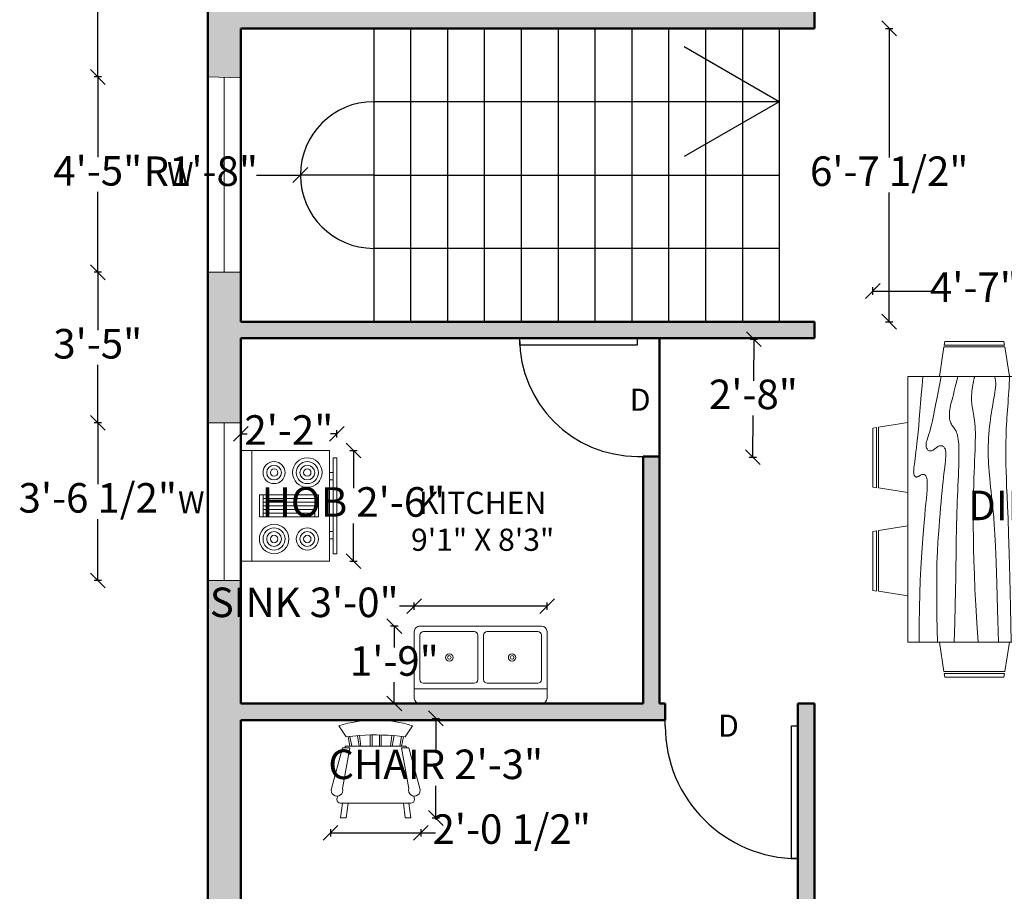
# Model space of a CAD drawing. Units: inches. Extents: x 2395 to 2921, y 528 to 1164.
# Tile 2 of 5: x 2395 to 2662, y 688 to 925. Entities that reach past the tile are written whole.
import ezdxf

# ---------------------------------------------------------------- set-up
doc = ezdxf.new("R2010")
doc.units = ezdxf.units.IN
for name, color, linetype, lineweight in [('A-ANNO-DIMS', 2, 'Continuous', 18), ('A-ANNO-TEXT', 7, 'Continuous', 18), ('A-AREA-IDEN', 7, 'Continuous', 25), ('A-DOOR', 3, 'Continuous', 25), ('A-EQPM', 9, 'Continuous', 18), ('A-FLOR-FIXT', 9, 'Continuous', 18), ('A-FLOR-STRS', 7, 'Continuous', 25), ('A-FURN', 8, 'Continuous', 18), ('A-GLAZ', 4, 'Continuous', 18), ('A-WALL', 162, 'Continuous', 50), ('A-WALL-PATT', 162, 'Continuous', 13)]:
    doc.layers.add(name, color=color, linetype=linetype, lineweight=lineweight)
doc.styles.get("Standard").update_dxf_attribs({"font": 'arial.ttf'})
doc.dimstyles.new('ISO-25', dxfattribs={"dimtxt": 8, "dimasz": 4, "dimexe": 1, "dimexo": 1, "dimtad": 0, "dimtih": 1, "dimtoh": 1, "dimlunit": 3, "dimtxsty": 'Standard', "dimblk": 'OBLIQUE', "dimcen": 2.5, "dimadec": 0, "dimazin": 0, "dimtfac": 1, "dimtmove": 0, "dimatfit": 3, "dimfxl": 1, "dimfxlon": 1, "dimarcsym": 0})

# ---------------------------------------------------------------- blocks, each defined once
blk = doc.blocks.new('*U9')
for p, q in [((0, 0), (0, -6)), ((-32, 0), (-32, -6))]:
    blk.add_line(p, q)
blk.add_lwpolyline([(0, 0), (0, 32), (-1.75, 32), (-1.75, 0)], close=True)
blk.add_arc((0, 0), 32, 90, 180)
blk = doc.blocks.new('*U5')
for p, q in [((-36, 0), (-36, 6)), ((0, 0), (0, 6))]:
    blk.add_line(p, q)
blk.add_lwpolyline([(0, 0), (0, -36), (-1.75, -36), (-1.75, 0)], close=True)
blk.add_arc((0, 0), 36, 180, 270)
blk = doc.blocks.new('Chair - Rocking')
for p, q in [((-8, -4.5), (-10, -1.5)), ((8, -4.5), (10, -1.5)), ((-7.5, -4.5), (-7, -7)), ((-6.5, -7), (-7.02225, -4.43)), ((-4.5, -7), (-4.96674, -4.19951)), ((-4, -7), (-4.40532, -4.16272)), ((-1.5, -4.05012), (-1.5, -7)), ((-1, -7), (-1, -4.05012)), ((1, -7), (1, -4.04655)), ((1.5, -4.05012), (1.5, -7)), ((4, -7), (4.40187, -4.18694)), ((4.5, -7), (4.96761, -4.19437)), ((6.5, -7), (7, -4.4057)), ((7.5, -4.5), (7, -7)), ((-9, -7.5), (-12, -18.49999)), ((-7, -7.5), (-9, -7.5)), ((-9, -18.49999), (-7, -7.5)), ((-8.23428, -6.99939), (-8.3093, -7.47958)), ((-8.23041, -7), (8.23915, -7)), ((7, -7.5), (9, -7.5)), ((9, -18.49999), (7, -7.5)), ((8.31071, -7.48854), (8.23449, -7.00073)), ((9, -7.5), (12, -18.49999)), ((-10.36644, -20.64523), (-10.5, -21.49999)), ((10.5, -21.49999), (10.3575, -20.58798)), ((-9, -22.49999), (-9.5, -26.49999)), ((0, -22.49999), (-9.5, -22.49999)), ((-8, -26.49999), (-7.5, -22.49999)), ((0, -22.49999), (9.5, -22.49999)), ((8, -26.49999), (7.5, -22.49999)), ((9, -22.49999), (9.5, -26.49999)), ((-9.5, -26.49999), (-8, -26.49999)), ((9.5, -26.49999), (8, -26.49999))]:
    blk.add_line(p, q)
for centre, radius, start, end in [((0, -34.08333), 34.08333, 72.93847, 107.0615), ((0, -68.25004), 64.25, 93.92211, 97.15267), ((0, -68.25004), 64.25, 82.84733, 93.92211), ((-10.5, -18.99999), 1.58114, 161.5651, 18.43495), ((10.5, -18.99999), 1.58114, 161.5651, 18.43495), ((-9.5, -21.49999), 1, 180, 270), ((9.5, -21.49999), 1, 270, 0)]:
    blk.add_arc(centre, radius, start, end)
blk = doc.blocks.new('Dining Set - 36 x 72 in.')
for p, q in [((-22, 27.5), (-22.1562, 26.50042)), ((-22, 27.5), (-6, 27.5)), ((-5.8437, 26.49966), (-6, 27.5)), ((6, 27.5), (5.8438, 26.50042)), ((6, 27.5), (22, 27.5)), ((22.1563, 26.49966), (22, 27.5)), ((-22.2343, 26.00059), (-23.4847, 17.99762)), ((-22.2304, 26), (-5.7608, 26)), ((-5.8416, 26.5), (-22.1534, 26.5)), ((-4.5152, 17.99762), (-5.7655, 25.99926)), ((5.7657, 26.00059), (4.5153, 17.99762)), ((5.7696, 26), (22.2392, 26)), ((22.1584, 26.5), (5.8466, 26.5)), ((23.4848, 17.99762), (22.2345, 25.99926)), ((36, 18), (-36, 18)), ((-36, 18), (-36, -18)), ((36, -18), (36, 18)), ((-45.5, 8), (-44.5004, 8.15617)), ((-44.5, -8.15843), (-44.5, 8.15338)), ((-44.0006, 8.23428), (-35.9976, 9.48474)), ((-44, 8.23041), (-44, -8.23915)), ((44.0006, 8.23428), (35.9976, 9.48474)), ((44, 8.23041), (44, -8.23915)), ((44.5, -8.15843), (44.5, 8.15338)), ((45.5, 8), (44.5005, 8.15617)), ((-45.5, 8), (-45.5, -8)), ((45.5, 8), (45.5, -8)), ((-44.4997, -8.15631), (-45.5, -8)), ((44.4997, -8.15631), (45.5, -8)), ((-35.9976, -9.48476), (-43.9993, -8.2345)), ((35.9976, -9.48476), (43.9993, -8.2345)), ((-36, -18), (36, -18)), ((-22.2343, -26.0006), (-23.4847, -17.99762)), ((-4.5152, -17.99762), (-5.7655, -25.99928)), ((5.7657, -26.0006), (4.5153, -17.99762)), ((23.4848, -17.99762), (22.2345, -25.99928)), ((-22.2304, -26), (-5.7608, -26)), ((-22, -27.5), (-22.1562, -26.50044)), ((-5.8416, -26.5), (-22.1534, -26.5)), ((-5.8437, -26.49967), (-6, -27.5)), ((5.7696, -26), (22.2392, -26)), ((6, -27.5), (5.8438, -26.50044)), ((22.1584, -26.5), (5.8466, -26.5)), ((22.1563, -26.49967), (22, -27.5)), ((-22, -27.5), (-6, -27.5)), ((6, -27.5), (22, -27.5))]:
    blk.add_line(p, q)
for points in [[(-36, 15), (-31.1772, 14.97754), (-26.8079, 14.91406), (-22.8538, 14.81543), (-19.276, 14.6875), (-16.0362, 14.53613), (-13.0957, 14.36718), (-10.4159, 14.18652), (-7.9583, 14), (-5.6904, 13.81315), (-3.6035, 13.63021), (-1.6954, 13.45508), (0.0365, 13.29166), (1.5945, 13.14388), (2.9811, 13.01562), (4.1988, 12.9108), (5.25, 12.83333), (6.1393, 12.78613), (6.8802, 12.76823), (7.4883, 12.77767), (7.9792, 12.8125), (8.3685, 12.87077), (8.6719, 12.95052), (8.9049, 13.0498), (9.0833, 13.16666), (9.2205, 13.29899), (9.3216, 13.44401), (9.3895, 13.59879), (9.4271, 13.76041), (9.4373, 13.92594), (9.4232, 14.09245), (9.3875, 14.257), (9.3333, 14.41666), (9.2638, 14.56917), (9.1836, 14.71484), (9.0975, 14.85465), (9.0104, 14.98958), (8.9272, 15.1206), (8.8529, 15.2487), (8.7922, 15.37483), (8.75, 15.5), (8.7305, 15.62467), (8.7344, 15.74739), (8.7617, 15.86621), (8.8125, 15.97916), (8.8867, 16.08431), (8.9844, 16.17968), (9.1055, 16.26334), (9.25, 16.33333), (9.4189, 16.38802), (9.6172, 16.42708), (9.8506, 16.45052), (10.125, 16.45833), (10.4463, 16.45052), (10.8203, 16.42708), (11.2529, 16.38802), (11.75, 16.33333), (12.3184, 16.26318), (12.9694, 16.17838), (13.7151, 16.07991), (14.5677, 15.96875), (15.5395, 15.84586), (16.6426, 15.71224), (17.8893, 15.56884), (19.2917, 15.41666), (20.859, 15.25667), (22.5879, 15.08984), (24.4721, 14.91715), (26.5052, 14.73958), (28.6809, 14.5581), (30.9929, 14.3737), (33.4347, 14.18733), (36, 14)], [(-36, 10), (-28.9766, 10.14274), (-23.1725, 10.20442), (-18.4241, 10.19775), (-14.5677, 10.13541), (-11.4399, 10.03011), (-8.877, 9.89453), (-6.7154, 9.74137), (-4.7917, 9.58333), (-2.9698, 9.43082), (-1.2246, 9.28515), (0.4415, 9.14534), (2.026, 9.01041), (3.5266, 8.87939), (4.9408, 8.7513), (6.266, 8.62516), (7.5, 8.5), (8.6411, 8.37549), (9.6914, 8.2539), (10.6538, 8.13818), (11.5312, 8.03125), (12.3267, 7.93603), (13.043, 7.85547), (13.6831, 7.79248), (14.25, 7.75), (14.7471, 7.7303), (15.1797, 7.73307), (15.5537, 7.75732), (15.875, 7.80208), (16.1494, 7.86637), (16.3828, 7.94922), (16.5811, 8.04964), (16.75, 8.16666), (16.8944, 8.29915), (17.0143, 8.44531), (17.1089, 8.60319), (17.1771, 8.77083), (17.218, 8.94629), (17.2305, 9.1276), (17.2137, 9.31282), (17.1667, 9.5), (17.0895, 9.6875), (16.987, 9.875), (16.8649, 10.0625), (16.7292, 10.25), (16.5856, 10.4375), (16.4401, 10.625), (16.2985, 10.8125), (16.1667, 11), (16.05, 11.18733), (15.9518, 11.3737), (15.8752, 11.5581), (15.8229, 11.73958), (15.798, 11.91715), (15.8034, 12.08984), (15.842, 12.25667), (15.9167, 12.41666), (16.0295, 12.56836), (16.1784, 12.70833), (16.3605, 12.83268), (16.5729, 12.9375), (16.8127, 13.01888), (17.0768, 13.07291), (17.3625, 13.0957), (17.6667, 13.08333), (17.9894, 13.03312), (18.3418, 12.94726), (18.7382, 12.82918), (19.1927, 12.68229), (19.7195, 12.51001), (20.3327, 12.31575), (21.0465, 12.10294), (21.875, 11.875), (22.8357, 11.63354), (23.959, 11.37304), (25.2786, 11.08618), (26.8282, 10.76562), (28.6414, 10.40405), (30.752, 9.99414), (33.1936, 9.52856), (36, 9)], [(-36, 5.5), (-30.7157, 5.3348), (-26.069, 5.20963), (-21.9946, 5.11767), (-18.4271, 5.05208), (-15.3009, 5.00602), (-12.5508, 4.97265), (-10.1112, 4.94515), (-7.9167, 4.91666), (-5.909, 4.88167), (-4.0586, 4.83984), (-2.3429, 4.79215), (-0.7396, 4.73958), (0.7739, 4.6831), (2.22, 4.6237), (3.6213, 4.56233), (5, 4.5), (6.373, 4.43782), (7.7344, 4.3776), (9.0723, 4.32129), (10.375, 4.27083), (11.6309, 4.22819), (12.8281, 4.19531), (13.9551, 4.17415), (15, 4.16666), (15.954, 4.17448), (16.819, 4.19791), (17.6001, 4.23698), (18.3021, 4.29166), (18.9299, 4.36198), (19.4883, 4.44791), (19.9823, 4.54948), (20.4167, 4.66666), (20.7969, 4.79899), (21.1302, 4.94401), (21.4245, 5.09879), (21.6875, 5.26041), (21.9271, 5.42594), (22.1511, 5.59245), (22.3672, 5.757), (22.5834, 5.91666), (22.8065, 6.06868), (23.0404, 6.21093), (23.2879, 6.34147), (23.5521, 6.45833), (23.8358, 6.55957), (24.142, 6.64323), (24.4735, 6.70735), (24.8334, 6.75), (25.2235, 6.76969), (25.642, 6.76692), (26.0858, 6.74267), (26.5521, 6.69791), (27.0379, 6.63362), (27.5404, 6.55078), (28.0565, 6.45036), (28.5834, 6.33333), (29.1242, 6.19987), (29.7071, 6.04687), (30.3661, 5.87044), (31.1354, 5.66666), (32.0493, 5.43164), (33.142, 5.16146), (34.4475, 4.85221), (36, 4.5)], [(-36, -1), (-30.7915, -0.6591), (-26.0195, -0.38216), (-21.6519, -0.16284), (-17.6563, 0.00521), (-14.0005, 0.12833), (-10.6523, 0.21289), (-7.5796, 0.26522), (-4.75, 0.29166), (-2.134, 0.29793), (0.2878, 0.28711), (2.5317, 0.26163), (4.6146, 0.22396), (6.5529, 0.17651), (8.3633, 0.12174), (10.0623, 0.06209), (11.6667, 0), (13.1899, -0.06201), (14.6341, -0.1211), (15.9982, -0.17432), (17.2813, -0.21875), (18.4823, -0.25147), (19.6003, -0.26953), (20.6343, -0.27002), (21.5834, -0.25), (22.4481, -0.20768), (23.2357, -0.14584), (23.9549, -0.06836), (24.6146, 0.02083), (25.2235, 0.11784), (25.7904, 0.21875), (26.3241, 0.31966), (26.8334, 0.41666), (27.3265, 0.50618), (27.8099, 0.58593), (28.2894, 0.65397), (28.7709, 0.70833), (29.2601, 0.74707), (29.763, 0.76823), (30.2855, 0.76985), (30.8334, 0.75), (31.4088, 0.70784), (31.9994, 0.64713), (32.589, 0.57275), (33.1615, 0.48958), (33.7008, 0.4025), (34.1908, 0.3164), (34.6153, 0.23616), (34.9584, 0.16666), (35.2099, 0.11165), (35.3848, 0.07031), (35.504, 0.04069), (35.5886, 0.02083), (35.6594, 0.00879), (35.7377, 0.0026), (35.8442, 0.00032), (36, 0)], [(-36, -6.5), (-27.1843, -6.31267), (-20.084, -6.1263), (-14.469, -5.9419), (-10.1094, -5.76042), (-6.7752, -5.58285), (-4.2363, -5.41016), (-2.2629, -5.24333), (-0.625, -5.08334), (0.8708, -4.93099), (2.2715, -4.78646), (3.5872, -4.64974), (4.8281, -4.52084), (6.0046, -4.39974), (7.127, -4.28646), (8.2053, -4.18099), (9.25, -4.08334), (10.2705, -3.99382), (11.2734, -3.91407), (12.2647, -3.84603), (13.25, -3.79167), (14.2354, -3.75293), (15.2266, -3.73177), (16.2295, -3.73015), (17.25, -3.75), (18.2912, -3.79248), (19.3451, -3.85547), (20.4009, -3.93604), (21.4479, -4.03125), (22.4754, -4.13819), (23.4727, -4.25391), (24.4289, -4.37549), (25.3334, -4.5), (26.1785, -4.62492), (26.9694, -4.74935), (27.7145, -4.87281), (28.4219, -4.99479), (29.1, -5.11483), (29.7572, -5.23242), (30.4016, -5.34709), (31.0417, -5.45834), (31.6837, -5.56437), (32.3262, -5.65821), (32.9658, -5.73153), (33.599, -5.77604), (34.2224, -5.78345), (34.8327, -5.74545), (35.4264, -5.65373), (36, -5.5)], [(-36, -10), (-26.4022, -9.81299), (-18.4675, -9.62891), (-11.9839, -9.45069), (-6.7396, -9.28125), (-2.5226, -9.12354), (0.8789, -8.98047), (3.6769, -8.85498), (6.0833, -8.75), (8.2767, -8.66765), (10.3021, -8.60677), (12.1712, -8.56543), (13.8958, -8.54167), (15.4876, -8.53353), (16.9583, -8.53907), (18.3197, -8.55632), (19.5834, -8.58334), (20.7616, -8.61841), (21.8685, -8.66081), (22.9188, -8.71004), (23.9271, -8.76563), (24.9081, -8.82707), (25.8763, -8.89388), (26.8465, -8.96558), (27.8334, -9.04167), (28.8474, -9.12118), (29.8828, -9.20117), (30.93, -9.27824), (31.9792, -9.34896), (33.0205, -9.40991), (34.0443, -9.45768), (35.0407, -9.48885), (36, -9.5)], [(-36, -14.5), (-30.0881, -14.33513), (-25.0332, -14.21224), (-20.7312, -14.12647), (-17.0781, -14.07292), (-13.97, -14.04671), (-11.3027, -14.04297), (-8.9724, -14.05681), (-6.875, -14.08334), (-4.9224, -14.11833), (-3.0905, -14.16016), (-1.3709, -14.20785), (0.2448, -14.26042), (1.7647, -14.3169), (3.1973, -14.3763), (4.5507, -14.43767), (5.8333, -14.5), (7.0554, -14.5621), (8.235, -14.62175), (9.3922, -14.67652), (10.5469, -14.72396), (11.7192, -14.76164), (12.929, -14.78711), (14.1965, -14.79794), (15.5417, -14.79167), (16.9933, -14.76424), (18.6152, -14.70508), (20.4804, -14.60197), (22.6615, -14.44271), (25.2312, -14.21509), (28.2624, -13.9069), (31.8277, -13.50594), (36, -13)]]:
    blk.add_lwpolyline(points)
blk = doc.blocks.new('Sink-double - 36 in top')
for p, q in [((-18, -4), (18, -4)), ((-0.75, -18.5), (-0.75, -6.5)), ((0.75, -6.5), (0.75, -18.5))]:
    blk.add_line(p, q)
for points in [[(-16.5, 0), (16.5, 0)], [(-18, -19.5), (-18, -1.5)], [(18, -1.5), (18, -19.5)], [(-16.5, -18.5), (-16.5, -6.5)], [(-15.5, -5.5), (-1.75, -5.5)], [(1.75, -5.5), (15.5, -5.5)], [(16.5, -6.5), (16.5, -18.5)], [(16.5, -21), (-16.5, -21)], [(-1.75, -19.5), (-15.5, -19.5)], [(15.5, -19.5), (1.75, -19.5)]]:
    blk.add_lwpolyline(points)
for centre, radius in [((-8.5, -12.5), 1), ((-8.5, -12.5), 0.5), ((8.5, -12.5), 1), ((8.5, -12.5), 0.5)]:
    blk.add_circle(centre, radius)
for centre, radius, start, end in [((-16.5, -1.5), 1.5, 90, 180), ((16.5, -1.5), 1.5, 0, 90), ((-15.5, -6.5), 1, 90, 180), ((-1.75, -6.5), 1, 0, 90), ((1.75, -6.5), 1, 90, 180), ((15.5, -6.5), 1, 0, 90), ((-15.5, -18.5), 1, 180, 270), ((-1.75, -18.5), 1, 270, 0), ((1.75, -18.5), 1, 180, 270), ((15.5, -18.5), 1, 270, 0), ((-16.5, -19.5), 1.5, 180, 270), ((16.5, -19.5), 1.5, 270, 0)]:
    blk.add_arc(centre, radius, start, end)
blk = doc.blocks.new('Range-Oven - 30 in top')
for p, q in [((0, -3), (30, -3)), ((12, -6), (18, -6)), ((13, -20), (13, -6)), ((14, -6), (14, -20)), ((15, -20), (15, -6)), ((16, -6), (16, -20)), ((17, -20), (17, -6)), ((18, -20), (12, -20)), ((6, -24), (6, -25)), ((8, -25), (8, -24)), ((22, -25), (22, -24)), ((24, -24), (24, -25))]:
    blk.add_line(p, q)
for points in [[(0, -24), (0, 0), (30, 0), (30, -24)], [(12, -21), (12, -5), (18, -5), (18, -21)], [(2, -26), (2, -25), (28, -25), (28, -26)]]:
    blk.add_lwpolyline(points, close=True)
for centre, radius in [((6, -9), 4), ((6, -9), 3), ((6, -9), 2), ((6, -9), 1), ((24, -9), 3), ((24, -9), 2), ((24, -9), 1), ((6, -18), 3), ((6, -18), 2), ((24, -18), 4), ((24, -18), 3), ((24, -18), 2), ((6, -18), 1), ((24, -18), 1)]:
    blk.add_circle(centre, radius)
blk = doc.blocks.new('_Oblique')
at = {"color": 0, "linetype": 'ByBlock', "lineweight": -2}
blk.add_line((-0.5, -0.5), (0.5, 0.5), dxfattribs=at)
blk = doc.blocks.new('*D30')
at = {"layer": 'A-ANNO-DIMS', "color": 0, "lineweight": -2, "transparency": 16777216}
for p, q in [((2507.01, 735.35), (2509.01, 735.35)), ((2508.01, 735.35), (2508.01, 726.62)), ((2508.01, 708.35), (2508.01, 717.09)), ((2507.01, 708.35), (2509.01, 708.35))]:
    blk.add_line(p, q, dxfattribs=at)
at = {"layer": 'Defpoints', "color": 0, "transparency": 16777216}
for p in [(2503.96, 735.35), (2508.01, 735.35), (2503.96, 708.35)]:
    blk.add_point(p, dxfattribs=at)
at = {"layer": 'A-ANNO-DIMS', "color": 0, "lineweight": -2, "transparency": 16777216, "xscale": 4, "yscale": 4, "zscale": 4}
for p, rotation in [((2508.01, 735.35), 90), ((2508.01, 708.35), 270)]:
    blk.add_blockref('_Oblique', p, dxfattribs=dict(at, rotation=rotation))
at = {"layer": 'A-ANNO-DIMS', "color": 0, "transparency": 16777216, "insert": (2508.01, 721.85), "char_height": 8, "attachment_point": 5}
blk.add_mtext('CHAIR 2\'-3"', dxfattribs=at)
blk = doc.blocks.new('*D31')
at = {"layer": 'A-ANNO-DIMS', "color": 0, "lineweight": -2, "transparency": 16777216}
for p, q in [((2479.52, 705.3), (2479.52, 703.3)), ((2503.96, 705.3), (2503.96, 703.3)), ((2479.52, 704.3), (2503.96, 704.3)), ((2503.96, 704.3), (2507.96, 704.3))]:
    blk.add_line(p, q, dxfattribs=at)
at = {"layer": 'Defpoints', "color": 0, "transparency": 16777216}
for p in [(2479.52, 708.35), (2503.96, 708.35), (2503.96, 704.3)]:
    blk.add_point(p, dxfattribs=at)
at = {"layer": 'A-ANNO-DIMS', "color": 0, "lineweight": -2, "transparency": 16777216, "xscale": 4, "yscale": 4, "zscale": 4, "rotation": 180}
blk.add_blockref('_Oblique', (2479.52, 704.3), dxfattribs=at)
at = {"layer": 'A-ANNO-DIMS', "color": 0, "lineweight": -2, "transparency": 16777216, "xscale": 4, "yscale": 4, "zscale": 4}
blk.add_blockref('_Oblique', (2503.96, 704.3), dxfattribs=at)
at = {"layer": 'A-ANNO-DIMS', "color": 0, "transparency": 16777216, "insert": (2528.6, 704.3), "char_height": 8, "attachment_point": 5}
blk.add_mtext('2\'-0 1/2"', dxfattribs=at)
blk = doc.blocks.new('*D36')
at = {"layer": 'A-ANNO-DIMS', "color": 0, "lineweight": -2, "transparency": 16777216}
for p, q in [((2694.16, 837.52), (2696.16, 837.52)), ((2695.16, 837.52), (2695.16, 796.78)), ((2695.16, 746.52), (2695.16, 787.26)), ((2694.16, 746.52), (2696.16, 746.52))]:
    blk.add_line(p, q, dxfattribs=at)
at = {"layer": 'Defpoints', "color": 0, "transparency": 16777216}
for p in [(2681.51, 837.52), (2695.16, 837.52), (2681.51, 746.52)]:
    blk.add_point(p, dxfattribs=at)
at = {"layer": 'A-ANNO-DIMS', "color": 0, "lineweight": -2, "transparency": 16777216, "xscale": 4, "yscale": 4, "zscale": 4}
for p, rotation in [((2695.16, 837.52), 90), ((2695.16, 746.52), 270)]:
    blk.add_blockref('_Oblique', p, dxfattribs=dict(at, rotation=rotation))
at = {"layer": 'A-ANNO-DIMS', "color": 0, "transparency": 16777216, "insert": (2695.16, 792.02), "char_height": 8, "attachment_point": 5}
blk.add_mtext('DINING SET 7\'-7"', dxfattribs=at)
blk = doc.blocks.new('*D37')
at = {"layer": 'A-ANNO-DIMS', "color": 0, "lineweight": -2, "transparency": 16777216}
for p, q in [((2626.51, 850.17), (2626.51, 852.17)), ((2681.51, 850.17), (2681.51, 852.17)), ((2626.51, 851.17), (2642.59, 851.17)), ((2681.51, 851.17), (2665.43, 851.17))]:
    blk.add_line(p, q, dxfattribs=at)
at = {"layer": 'Defpoints', "color": 0, "transparency": 16777216}
for p in [(2626.51, 851.17), (2626.51, 837.52), (2681.51, 837.52)]:
    blk.add_point(p, dxfattribs=at)
at = {"layer": 'A-ANNO-DIMS', "color": 0, "lineweight": -2, "transparency": 16777216, "xscale": 4, "yscale": 4, "zscale": 4, "rotation": 180}
blk.add_blockref('_Oblique', (2626.51, 851.17), dxfattribs=at)
at = {"layer": 'A-ANNO-DIMS', "color": 0, "lineweight": -2, "transparency": 16777216, "xscale": 4, "yscale": 4, "zscale": 4}
blk.add_blockref('_Oblique', (2681.51, 851.17), dxfattribs=at)
at = {"layer": 'A-ANNO-DIMS', "color": 0, "transparency": 16777216, "insert": (2654.01, 851.17), "char_height": 8, "attachment_point": 5}
blk.add_mtext('4\'-7"', dxfattribs=at)
blk = doc.blocks.new('*D38')
at = {"layer": 'A-ANNO-DIMS', "color": 0, "lineweight": -2, "transparency": 16777216}
for p, q in [((2502.19, 764.75), (2502.19, 766.75)), ((2538.19, 764.75), (2538.19, 766.75)), ((2502.19, 765.75), (2498.19, 765.75)), ((2538.19, 765.75), (2502.19, 765.75))]:
    blk.add_line(p, q, dxfattribs=at)
at = {"layer": 'Defpoints', "color": 0, "transparency": 16777216}
for p in [(2502.19, 765.75), (2502.19, 760.35), (2538.19, 760.35)]:
    blk.add_point(p, dxfattribs=at)
at = {"layer": 'A-ANNO-DIMS', "color": 0, "lineweight": -2, "transparency": 16777216, "xscale": 4, "yscale": 4, "zscale": 4, "rotation": 180}
blk.add_blockref('_Oblique', (2502.19, 765.75), dxfattribs=at)
at = {"layer": 'A-ANNO-DIMS', "color": 0, "lineweight": -2, "transparency": 16777216, "xscale": 4, "yscale": 4, "zscale": 4}
blk.add_blockref('_Oblique', (2538.19, 765.75), dxfattribs=at)
at = {"layer": 'A-ANNO-DIMS', "color": 0, "transparency": 16777216, "insert": (2472.36, 765.75), "char_height": 8, "attachment_point": 5}
blk.add_mtext('SINK 3\'-0"', dxfattribs=at)
blk = doc.blocks.new('*D39')
at = {"layer": 'A-ANNO-DIMS', "color": 0, "lineweight": -2, "transparency": 16777216}
for p, q in [((2497.79, 760.35), (2495.79, 760.35)), ((2496.79, 760.35), (2496.79, 754.56)), ((2496.79, 739.35), (2496.79, 745.14)), ((2497.79, 739.35), (2495.79, 739.35))]:
    blk.add_line(p, q, dxfattribs=at)
at = {"layer": 'Defpoints', "color": 0, "transparency": 16777216}
for p in [(2502.19, 760.35), (2496.79, 739.35), (2502.19, 739.35)]:
    blk.add_point(p, dxfattribs=at)
at = {"layer": 'A-ANNO-DIMS', "color": 0, "lineweight": -2, "transparency": 16777216, "xscale": 4, "yscale": 4, "zscale": 4}
for p, rotation in [((2496.79, 760.35), 90), ((2496.79, 739.35), 270)]:
    blk.add_blockref('_Oblique', p, dxfattribs=dict(at, rotation=rotation))
at = {"layer": 'A-ANNO-DIMS', "color": 0, "transparency": 16777216, "insert": (2496.79, 749.85), "char_height": 8, "attachment_point": 5}
blk.add_mtext('1\'-9"', dxfattribs=at)
blk = doc.blocks.new('*D40')
at = {"layer": 'A-ANNO-DIMS', "color": 0, "lineweight": -2, "transparency": 16777216}
for p, q in [((2484.7, 807.96), (2486.7, 807.96)), ((2485.7, 807.96), (2485.7, 797.73)), ((2485.7, 777.96), (2485.7, 788.2)), ((2484.7, 777.96), (2486.7, 777.96))]:
    blk.add_line(p, q, dxfattribs=at)
at = {"layer": 'Defpoints', "color": 0, "transparency": 16777216}
for p in [(2481.2, 807.96), (2485.7, 807.96), (2481.2, 777.96)]:
    blk.add_point(p, dxfattribs=at)
at = {"layer": 'A-ANNO-DIMS', "color": 0, "lineweight": -2, "transparency": 16777216, "xscale": 4, "yscale": 4, "zscale": 4}
for p, rotation in [((2485.7, 807.96), 90), ((2485.7, 777.96), 270)]:
    blk.add_blockref('_Oblique', p, dxfattribs=dict(at, rotation=rotation))
at = {"layer": 'A-ANNO-DIMS', "color": 0, "transparency": 16777216, "insert": (2485.7, 792.96), "char_height": 8, "attachment_point": 5}
blk.add_mtext('HOB 2\'-6"', dxfattribs=at)
blk = doc.blocks.new('*D41')
at = {"layer": 'A-ANNO-DIMS', "color": 0, "lineweight": -2, "transparency": 16777216}
for p, q in [((2455.2, 811.46), (2455.2, 813.46)), ((2455.2, 812.46), (2456.87, 812.46)), ((2481.2, 812.46), (2479.53, 812.46)), ((2481.2, 811.46), (2481.2, 813.46))]:
    blk.add_line(p, q, dxfattribs=at)
at = {"layer": 'Defpoints', "color": 0, "transparency": 16777216}
for p in [(2455.2, 812.46), (2455.2, 807.96), (2481.2, 807.96)]:
    blk.add_point(p, dxfattribs=at)
at = {"layer": 'A-ANNO-DIMS', "color": 0, "lineweight": -2, "transparency": 16777216, "xscale": 4, "yscale": 4, "zscale": 4, "rotation": 180}
blk.add_blockref('_Oblique', (2455.2, 812.46), dxfattribs=at)
at = {"layer": 'A-ANNO-DIMS', "color": 0, "lineweight": -2, "transparency": 16777216, "xscale": 4, "yscale": 4, "zscale": 4}
blk.add_blockref('_Oblique', (2481.2, 812.46), dxfattribs=at)
at = {"layer": 'A-ANNO-DIMS', "color": 0, "transparency": 16777216, "insert": (2468.2, 812.46), "char_height": 8, "attachment_point": 5}
blk.add_mtext('2\'-2"', dxfattribs=at)
blk = doc.blocks.new('*D51')
at = {"layer": 'A-ANNO-DIMS', "color": 0, "lineweight": -2, "transparency": 16777216}
for p, q in [((2606.2, 1150.65), (2606.2, 1152.65)), ((2606.2, 1151.65), (2610.7, 1151.65)), ((2610.7, 1150.65), (2610.7, 1152.65)), ((2610.7, 1151.65), (2614.7, 1151.65))]:
    blk.add_line(p, q, dxfattribs=at)
at = {"layer": 'Defpoints', "color": 0, "transparency": 16777216}
for p in [(2610.7, 1151.65), (2606.2, 578.85), (2610.7, 578.85)]:
    blk.add_point(p, dxfattribs=at)
at = {"layer": 'A-ANNO-DIMS', "color": 0, "lineweight": -2, "transparency": 16777216, "xscale": 4, "yscale": 4, "zscale": 4, "rotation": 180}
blk.add_blockref('_Oblique', (2606.2, 1151.65), dxfattribs=at)
at = {"layer": 'A-ANNO-DIMS', "color": 0, "lineweight": -2, "transparency": 16777216, "xscale": 4, "yscale": 4, "zscale": 4}
blk.add_blockref('_Oblique', (2610.7, 1151.65), dxfattribs=at)
at = {"layer": 'A-ANNO-DIMS', "color": 0, "transparency": 16777216, "insert": (2635.28, 1151.65), "char_height": 8, "attachment_point": 5}
blk.add_mtext('0\'-4 1/2"', dxfattribs=at)
blk = doc.blocks.new('*D52')
at = {"layer": 'A-ANNO-DIMS', "color": 0, "lineweight": -2, "transparency": 16777216}
for p, q in [((2629.93, 922.35), (2631.93, 922.35)), ((2630.93, 922.35), (2630.93, 887.36)), ((2630.93, 842.85), (2630.93, 877.84)), ((2629.93, 842.85), (2631.93, 842.85))]:
    blk.add_line(p, q, dxfattribs=at)
at = {"layer": 'Defpoints', "color": 0, "transparency": 16777216}
for p in [(2601.13, 922.35), (2601.13, 842.85), (2630.93, 842.85)]:
    blk.add_point(p, dxfattribs=at)
at = {"layer": 'A-ANNO-DIMS', "color": 0, "lineweight": -2, "transparency": 16777216, "xscale": 4, "yscale": 4, "zscale": 4}
for p, rotation in [((2630.93, 922.35), 90), ((2630.93, 842.85), 270)]:
    blk.add_blockref('_Oblique', p, dxfattribs=dict(at, rotation=rotation))
at = {"layer": 'A-ANNO-DIMS', "color": 0, "transparency": 16777216, "insert": (2630.93, 882.6), "char_height": 8, "attachment_point": 5}
blk.add_mtext('6\'-7 1/2"', dxfattribs=at)
blk = doc.blocks.new('*D53')
at = {"layer": 'A-ANNO-DIMS', "color": 0, "lineweight": -2, "transparency": 16777216}
for p, q in [((2455.2, 1150.65), (2455.2, 1152.65)), ((2455.2, 1151.65), (2461.94, 1151.65)), ((2491.2, 1151.65), (2484.46, 1151.65)), ((2491.2, 1150.65), (2491.2, 1152.65))]:
    blk.add_line(p, q, dxfattribs=at)
at = {"layer": 'Defpoints', "color": 0, "transparency": 16777216}
for p in [(2491.2, 1151.65), (2455.2, 922.35), (2491.2, 922.35)]:
    blk.add_point(p, dxfattribs=at)
at = {"layer": 'A-ANNO-DIMS', "color": 0, "lineweight": -2, "transparency": 16777216, "xscale": 4, "yscale": 4, "zscale": 4, "rotation": 180}
blk.add_blockref('_Oblique', (2455.2, 1151.65), dxfattribs=at)
at = {"layer": 'A-ANNO-DIMS', "color": 0, "lineweight": -2, "transparency": 16777216, "xscale": 4, "yscale": 4, "zscale": 4}
blk.add_blockref('_Oblique', (2491.2, 1151.65), dxfattribs=at)
at = {"layer": 'A-ANNO-DIMS', "color": 0, "transparency": 16777216, "insert": (2473.2, 1151.65), "char_height": 8, "attachment_point": 5}
blk.add_mtext('3\'-0"', dxfattribs=at)
blk = doc.blocks.new('*D54')
at = {"layer": 'A-ANNO-DIMS', "color": 0, "lineweight": -2, "transparency": 16777216}
for p, q in [((2491.2, 1150.65), (2491.2, 1152.65)), ((2491.2, 1151.65), (2534.91, 1151.65)), ((2601.13, 1151.65), (2557.42, 1151.65)), ((2601.13, 1150.65), (2601.13, 1152.65))]:
    blk.add_line(p, q, dxfattribs=at)
at = {"layer": 'Defpoints', "color": 0, "transparency": 16777216}
for p in [(2601.13, 1151.65), (2491.2, 922.35), (2601.13, 922.35)]:
    blk.add_point(p, dxfattribs=at)
at = {"layer": 'A-ANNO-DIMS', "color": 0, "lineweight": -2, "transparency": 16777216, "xscale": 4, "yscale": 4, "zscale": 4, "rotation": 180}
blk.add_blockref('_Oblique', (2491.2, 1151.65), dxfattribs=at)
at = {"layer": 'A-ANNO-DIMS', "color": 0, "lineweight": -2, "transparency": 16777216, "xscale": 4, "yscale": 4, "zscale": 4}
blk.add_blockref('_Oblique', (2601.13, 1151.65), dxfattribs=at)
at = {"layer": 'A-ANNO-DIMS', "color": 0, "transparency": 16777216, "insert": (2546.16, 1151.65), "char_height": 8, "attachment_point": 5}
blk.add_mtext('9\'-2"', dxfattribs=at)
blk = doc.blocks.new('*D55')
at = {"layer": 'A-ANNO-DIMS', "color": 0, "lineweight": -2, "transparency": 16777216}
for p, q in [((2491.2, 1150.65), (2491.2, 1152.65)), ((2491.2, 1151.65), (2501.19, 1151.65)), ((2501.19, 1150.65), (2501.19, 1152.65)), ((2501.19, 1151.65), (2505.19, 1151.65))]:
    blk.add_line(p, q, dxfattribs=at)
at = {"layer": 'Defpoints', "color": 0, "transparency": 16777216}
for p in [(2501.19, 1151.65), (2491.2, 842.85), (2501.19, 842.85)]:
    blk.add_point(p, dxfattribs=at)
at = {"layer": 'A-ANNO-DIMS', "color": 0, "lineweight": -2, "transparency": 16777216, "xscale": 4, "yscale": 4, "zscale": 4, "rotation": 180}
blk.add_blockref('_Oblique', (2491.2, 1151.65), dxfattribs=at)
at = {"layer": 'A-ANNO-DIMS', "color": 0, "lineweight": -2, "transparency": 16777216, "xscale": 4, "yscale": 4, "zscale": 4}
blk.add_blockref('_Oblique', (2501.19, 1151.65), dxfattribs=at)
at = {"layer": 'A-ANNO-DIMS', "color": 0, "transparency": 16777216, "insert": (2519.56, 1151.65), "char_height": 8, "attachment_point": 5}
blk.add_mtext('0\'-10"', dxfattribs=at)
blk = doc.blocks.new('*D58')
at = {"layer": 'A-ANNO-DIMS', "color": 0, "lineweight": -2, "transparency": 16777216}
for p, q in [((2417.4, 997.65), (2415.4, 997.65)), ((2416.4, 997.65), (2416.4, 958.18)), ((2416.4, 909.18), (2416.4, 948.66)), ((2417.4, 909.18), (2415.4, 909.18))]:
    blk.add_line(p, q, dxfattribs=at)
at = {"layer": 'Defpoints', "color": 0, "transparency": 16777216}
for p in [(2446.2, 997.65), (2416.4, 909.18), (2446.2, 909.18)]:
    blk.add_point(p, dxfattribs=at)
at = {"layer": 'A-ANNO-DIMS', "color": 0, "lineweight": -2, "transparency": 16777216, "xscale": 4, "yscale": 4, "zscale": 4}
for p, rotation in [((2416.4, 997.65), 90), ((2416.4, 909.18), 270)]:
    blk.add_blockref('_Oblique', p, dxfattribs=dict(at, rotation=rotation))
at = {"layer": 'A-ANNO-DIMS', "color": 0, "transparency": 16777216, "insert": (2416.4, 953.42), "char_height": 8, "attachment_point": 5}
blk.add_mtext('7\'-4 1/2"', dxfattribs=at)
blk = doc.blocks.new('*D59')
at = {"layer": 'A-ANNO-DIMS', "color": 0, "lineweight": -2, "transparency": 16777216}
for p, q in [((2417.4, 909.18), (2415.4, 909.18)), ((2416.4, 909.18), (2416.4, 887.4)), ((2416.4, 856.24), (2416.4, 878.02)), ((2417.4, 856.24), (2415.4, 856.24))]:
    blk.add_line(p, q, dxfattribs=at)
at = {"layer": 'Defpoints', "color": 0, "transparency": 16777216}
for p in [(2446.2, 909.18), (2416.4, 856.24), (2446.2, 856.24)]:
    blk.add_point(p, dxfattribs=at)
at = {"layer": 'A-ANNO-DIMS', "color": 0, "lineweight": -2, "transparency": 16777216, "xscale": 4, "yscale": 4, "zscale": 4}
for p, rotation in [((2416.4, 909.18), 90), ((2416.4, 856.24), 270)]:
    blk.add_blockref('_Oblique', p, dxfattribs=dict(at, rotation=rotation))
at = {"layer": 'A-ANNO-DIMS', "color": 0, "transparency": 16777216, "insert": (2416.4, 882.71), "char_height": 8, "attachment_point": 5}
blk.add_mtext('4\'-5"', dxfattribs=at)
blk = doc.blocks.new('*D60')
at = {"layer": 'A-ANNO-DIMS', "color": 0, "lineweight": -2, "transparency": 16777216}
for p, q in [((2417.4, 856.24), (2415.4, 856.24)), ((2416.4, 856.24), (2416.4, 840.54)), ((2416.4, 815.43), (2416.4, 831.12)), ((2417.4, 815.43), (2415.4, 815.43))]:
    blk.add_line(p, q, dxfattribs=at)
at = {"layer": 'Defpoints', "color": 0, "transparency": 16777216}
for p in [(2446.2, 856.24), (2416.4, 815.43), (2446.2, 815.43)]:
    blk.add_point(p, dxfattribs=at)
at = {"layer": 'A-ANNO-DIMS', "color": 0, "lineweight": -2, "transparency": 16777216, "xscale": 4, "yscale": 4, "zscale": 4}
for p, rotation in [((2416.4, 856.24), 90), ((2416.4, 815.43), 270)]:
    blk.add_blockref('_Oblique', p, dxfattribs=dict(at, rotation=rotation))
at = {"layer": 'A-ANNO-DIMS', "color": 0, "transparency": 16777216, "insert": (2416.4, 835.83), "char_height": 8, "attachment_point": 5}
blk.add_mtext('3\'-5"', dxfattribs=at)
blk = doc.blocks.new('*D61')
at = {"layer": 'A-ANNO-DIMS', "color": 0, "lineweight": -2, "transparency": 16777216}
for p, q in [((2417.4, 815.43), (2415.4, 815.43)), ((2416.4, 815.43), (2416.4, 798.83)), ((2416.4, 772.71), (2416.4, 789.3)), ((2417.4, 772.71), (2415.4, 772.71))]:
    blk.add_line(p, q, dxfattribs=at)
at = {"layer": 'Defpoints', "color": 0, "transparency": 16777216}
for p in [(2446.2, 815.43), (2416.4, 772.71), (2446.2, 772.71)]:
    blk.add_point(p, dxfattribs=at)
at = {"layer": 'A-ANNO-DIMS', "color": 0, "lineweight": -2, "transparency": 16777216, "xscale": 4, "yscale": 4, "zscale": 4}
for p, rotation in [((2416.4, 815.43), 90), ((2416.4, 772.71), 270)]:
    blk.add_blockref('_Oblique', p, dxfattribs=dict(at, rotation=rotation))
at = {"layer": 'A-ANNO-DIMS', "color": 0, "transparency": 16777216, "insert": (2416.4, 794.07), "char_height": 8, "attachment_point": 5}
blk.add_mtext('3\'-6 1/2"', dxfattribs=at)
blk = doc.blocks.new('*D77')
at = {"layer": 'A-ANNO-DIMS', "color": 0, "lineweight": -2, "transparency": 16777216}
for p, q in [((2593.25, 838.13), (2595.25, 838.11)), ((2594.25, 838.12), (2594.16, 826.83)), ((2594, 806.12), (2594.09, 817.41)), ((2593, 806.13), (2595, 806.11))]:
    blk.add_line(p, q, dxfattribs=at)
at = {"layer": 'Defpoints', "color": 0, "transparency": 16777216}
for p in [(2564.45, 838.35), (2564.2, 806.35), (2594, 806.12)]:
    blk.add_point(p, dxfattribs=at)
at = {"layer": 'A-ANNO-DIMS', "color": 0, "lineweight": -2, "transparency": 16777216, "xscale": 4, "yscale": 4, "zscale": 4}
for p, rotation in [((2594.25, 838.12), 89.55238582914113), ((2594, 806.12), 269.5523858291411)]:
    blk.add_blockref('_Oblique', p, dxfattribs=dict(at, rotation=rotation))
at = {"layer": 'A-ANNO-DIMS', "color": 0, "transparency": 16777216, "insert": (2594.12, 822.12), "char_height": 8, "attachment_point": 5}
blk.add_mtext('2\'-8"', dxfattribs=at)
blk = doc.blocks.new('*D78')
at = {"layer": 'A-ANNO-DIMS', "color": 0, "lineweight": -2, "transparency": 16777216}
for p, q in [((2570.2, 1150.65), (2570.2, 1152.65)), ((2570.2, 1151.65), (2576.94, 1151.65)), ((2606.2, 1151.65), (2599.46, 1151.65)), ((2606.2, 1150.65), (2606.2, 1152.65))]:
    blk.add_line(p, q, dxfattribs=at)
at = {"layer": 'Defpoints', "color": 0, "transparency": 16777216}
for p in [(2606.2, 1151.65), (2570.2, 734.85), (2606.2, 735.1)]:
    blk.add_point(p, dxfattribs=at)
at = {"layer": 'A-ANNO-DIMS', "color": 0, "lineweight": -2, "transparency": 16777216, "xscale": 4, "yscale": 4, "zscale": 4, "rotation": 180}
blk.add_blockref('_Oblique', (2570.2, 1151.65), dxfattribs=at)
at = {"layer": 'A-ANNO-DIMS', "color": 0, "lineweight": -2, "transparency": 16777216, "xscale": 4, "yscale": 4, "zscale": 4}
blk.add_blockref('_Oblique', (2606.2, 1151.65), dxfattribs=at)
at = {"layer": 'A-ANNO-DIMS', "color": 0, "transparency": 16777216, "insert": (2588.2, 1151.65), "char_height": 8, "attachment_point": 5}
blk.add_mtext('3\'-0"', dxfattribs=at)
blk = doc.blocks.new('*D80')
at = {"layer": 'A-ANNO-DIMS', "color": 0, "lineweight": -2, "transparency": 16777216}
for p in [(2459.4, 882.6), (2491.2, 882.6)]:
    blk.add_line(p, (2471.32, 882.6), dxfattribs=at)
at = {"layer": 'Defpoints', "color": 0, "transparency": 16777216}
for p in [(2471.32, 882.6), (2491.2, 882.6)]:
    blk.add_point(p, dxfattribs=at)
at = {"layer": 'A-ANNO-DIMS', "color": 0, "lineweight": -2, "transparency": 16777216, "xscale": 4, "yscale": 4, "zscale": 4, "rotation": 0.0088732788324949}
blk.add_blockref('_Oblique', (2471.32, 882.6), dxfattribs=at)
at = {"layer": 'A-ANNO-DIMS', "color": 0, "transparency": 16777216, "insert": (2444.31, 882.6), "char_height": 8, "attachment_point": 5}
blk.add_mtext('R1\'-8"', dxfattribs=at)

msp = doc.modelspace()

# ---------------------------------------------------------------- hatches: boundary and pattern name
at = {"layer": 'A-WALL-PATT'}
h = msp.add_hatch(color=256, dxfattribs=at)
h.dxf.hatch_style = 1
h.paths.add_polyline_path([(2627.2, 1121.853), (2446.2, 1121.853), (2446.2, 1054.648), (2455.2, 1054.648), (2455.2, 1112.853), (2606.2, 1112.853), (2606.2, 1022.853), (2610.7, 1022.853), (2610.7, 1112.853), (2627.2, 1112.853)])
h.paths.add_polyline_path([(2685.7, 1121.853), (2648.2, 1121.853), (2648.2, 1112.853), (2664.7, 1112.853), (2664.7, 992.853), (2606.2, 992.853), (2606.2, 962.853), (2610.7, 962.853), (2610.7, 988.353), (2669.2, 988.353), (2669.2, 994.353), (2669.2, 1024.353), (2669.2, 1112.853), (2685.7, 1112.853)])
h.paths.add_polyline_path([(2866.2, 1121.853), (2706.7, 1121.853), (2706.7, 1112.853), (2723.2, 1112.853), (2723.2, 992.853), (2699.2, 992.853), (2699.2, 988.353), (2723.2, 988.353), (2723.2, 962.853), (2727.7, 962.853), (2727.7, 1112.853), (2857.2, 1112.853), (2857.2, 1049.508), (2866.2, 1049.508)])
h.paths.add_polyline_path([(2866.2, 985.129), (2857.2, 985.129), (2857.2, 926.853), (2723.2, 926.853), (2723.2, 922.353), (2729.2, 922.353), (2765.2, 922.353), (2857.2, 922.353), (2857.2, 894.873), (2866.2, 894.873)])
h.paths.add_polyline_path([(2455.2, 997.652), (2446.2, 997.652), (2446.2, 909.181), (2455.2, 908.938), (2455.2, 922.353), (2610.7, 922.353), (2610.7, 926.853), (2455.2, 926.853)])
h.paths.add_polyline_path([(2455.2, 838.353), (2610.7, 838.353), (2610.7, 842.853), (2455.2, 842.853), (2455.2, 856.236), (2446.2, 856.236), (2446.2, 815.427), (2455.2, 815.427)])
h.paths.add_polyline_path([(2455.2, 772.706), (2446.2, 772.706), (2446.2, 569.853), (2505.031, 569.853), (2505.031, 578.853), (2455.2, 578.853), (2455.2, 734.853), (2570.2, 734.853), (2570.2, 739.353), (2568.7, 739.353), (2568.7, 806.353), (2564.2, 806.353), (2564.2, 739.353), (2455.2, 739.353)])
h.paths.add_polyline_path([(2656.2, 578.853), (2610.7, 578.853), (2610.7, 739.353), (2606.2, 739.353), (2606.2, 578.853), (2565.031, 578.853), (2565.031, 569.853), (2656.2, 569.853)])
h.paths.add_polyline_path([(2733.198, 578.853), (2716.2, 578.853), (2716.2, 569.853), (2733.198, 569.853)])
h.paths.add_polyline_path([(2801.188, 578.853), (2764.893, 578.853), (2764.893, 569.853), (2801.188, 569.853)])
h.paths.add_polyline_path([(2866.2, 616.306), (2857.2, 616.306), (2857.2, 578.853), (2836.314, 578.853), (2836.314, 569.853), (2866.2, 569.853)])
h.paths.add_polyline_path([(2866.2, 727.906), (2857.2, 727.906), (2857.2, 670.095), (2866.2, 670.095)])
h.paths.add_polyline_path([(2866.2, 831.149), (2857.2, 831.149), (2857.2, 795.353), (2727.7, 795.353), (2727.7, 886.353), (2723.2, 886.353), (2723.2, 790.853), (2857.2, 790.853), (2857.2, 777.101), (2866.2, 777.101)])

# ---------------------------------------------------------------- linework, layer by layer
at = {"layer": 'A-FLOR-STRS'}
for p, q in [((2491.2, 922.353), (2491.2, 842.853)), ((2501.193, 922.353), (2501.193, 842.853)), ((2511.187, 922.353), (2511.187, 842.853)), ((2521.18, 922.353), (2521.18, 842.853)), ((2531.173, 922.353), (2531.173, 842.853)), ((2541.167, 922.353), (2541.167, 842.853)), ((2551.16, 922.353), (2551.16, 842.853)), ((2561.153, 922.353), (2561.153, 842.853)), ((2571.147, 922.353), (2571.147, 842.853)), ((2581.14, 922.353), (2581.14, 842.853)), ((2591.133, 922.353), (2591.133, 842.853)), ((2601.127, 922.353), (2601.127, 842.853)), ((2601.127, 902.478), (2575.341, 917.365)), ((2601.127, 902.478), (2491.2, 902.478)), ((2601.127, 902.478), (2575.341, 887.591)), ((2491.2, 882.603), (2601.127, 882.603)), ((2601.127, 862.728), (2491.2, 862.728))]:
    msp.add_line(p, q, dxfattribs=at)
msp.add_arc((2491.2, 882.603), 19.875, 90, 270, dxfattribs=at)
at = {"layer": 'A-GLAZ'}
for p, q in [((2455.2, 908.938), (2446.2, 909.181)), ((2450.7, 856.236), (2450.7, 909.06)), ((2455.2, 856.236), (2446.2, 856.236)), ((2455.2, 815.427), (2446.2, 815.427)), ((2450.7, 815.427), (2450.7, 772.706)), ((2455.2, 772.706), (2446.2, 772.706))]:
    msp.add_line(p, q, dxfattribs=at)
at = {"layer": 'A-WALL'}
for p, q in [((2446.2, 1121.853), (2446.2, 569.853)), ((2610.7, 926.853), (2610.7, 922.353)), ((2455.2, 922.353), (2610.7, 922.353)), ((2455.2, 922.353), (2455.2, 842.853)), ((2610.7, 842.853), (2455.2, 842.853)), ((2610.7, 838.353), (2610.7, 842.853)), ((2455.2, 838.353), (2455.2, 739.353)), ((2610.7, 838.353), (2455.2, 838.353)), ((2568.7, 838.353), (2568.7, 739.353)), ((2564.2, 806.353), (2564.2, 739.353)), ((2568.7, 806.353), (2564.2, 806.353)), ((2564.2, 739.353), (2455.2, 739.353)), ((2570.2, 739.353), (2568.7, 739.353)), ((2570.2, 739.353), (2570.2, 734.853)), ((2606.2, 578.853), (2606.2, 739.353)), ((2610.7, 739.353), (2606.2, 739.353)), ((2610.7, 578.853), (2610.7, 739.353)), ((2570.2, 734.853), (2455.2, 734.853)), ((2455.2, 734.853), (2455.2, 578.853))]:
    msp.add_line(p, q, dxfattribs=at)

# ---------------------------------------------------------------- block references
at = {"layer": 'A-DOOR', "rotation": 90}
msp.add_blockref('*U9', (2562.7, 838.353), dxfattribs=at)
at = {"layer": 'A-DOOR'}
msp.add_blockref('*U5', (2606.2, 733.353), dxfattribs=at)
at = {"layer": 'A-EQPM', "rotation": 90}
msp.add_blockref('Range-Oven - 30 in top', (2455.2, 777.961), dxfattribs=at)
at = {"layer": 'A-FLOR-FIXT', "rotation": 180}
msp.add_blockref('Sink-double - 36 in top', (2520.194, 739.353), dxfattribs=at)
at = {"layer": 'A-FURN', "rotation": 90}
msp.add_blockref('Dining Set - 36 x 72 in.', (2654.008, 792.019), dxfattribs=at)
at = {"layer": 'A-FURN'}
msp.add_blockref('Chair - Rocking', (2491.739, 734.853), dxfattribs=at)

# ---------------------------------------------------------------- texts
at = {"layer": 'A-ANNO-TEXT', "char_height": 6, "attachment_point": 1}
for s, insert in [('\\pxqc;W', (2432.557, 886.128)), ('\\pxqc;D', (2557.207, 824.696)), ('\\pxqc;W', (2435.534, 796.917)), ('\\pxqc;D', (2581.146, 736.359))]:
    msp.add_mtext_dynamic_manual_height_columns(s, width=12.42697, gutter_width=12.5, heights=[0], dxfattribs=dict(at, insert=insert))
at = {"layer": 'A-AREA-IDEN', "insert": (2500.736, 796.753), "char_height": 6, "attachment_point": 1}
msp.add_mtext_dynamic_manual_height_columns('\\pxqc;KITCHEN\\P9\'1" X 8\'3"', width=39.98375, gutter_width=12.5, heights=[0], dxfattribs=at)

# ---------------------------------------------------------------- dimensions: what is measured, and where the dimension line sits
at = {"layer": 'A-ANNO-DIMS'}
for base, p1, p2, picture, middle in [((2610.7, 1151.653), (2606.2, 578.853), (2610.7, 578.853), '*D51', (2635.278, 1151.653)), ((2491.2, 1151.653), (2455.2, 922.353), (2491.2, 922.353), '*D53', (2473.2, 1151.653)), ((2601.127, 1151.653), (2491.2, 922.353), (2601.127, 922.353), '*D54', (2546.163, 1151.653)), ((2501.193, 1151.653), (2491.2, 842.853), (2501.193, 842.853), '*D55', (2519.559, 1151.653)), ((2606.2, 1151.653), (2570.2, 734.853), (2606.2, 735.103), '*D78', (2588.2, 1151.653)), ((2503.956, 704.303), (2479.521, 708.353), (2503.956, 708.353), '*D31', (2528.603, 704.303))]:
    dim = msp.add_linear_dim(base=base, p1=p1, p2=p2, dimstyle='ISO-25', override={"dimdec": 1, "dimlfac": 1, "dimrnd": 0, "dimzin": 1, "dimdsep": 46, "dimlunit": 4, "dimfrac": 2}, dxfattribs=at)
    dim.commit()
    dim.dimension.update_dxf_attribs({"geometry": picture, "text_midpoint": middle})
for base, p1, p2, angle, picture, middle in [((2416.4, 909.181), (2446.2, 997.652), (2446.2, 909.181), 90, '*D58', (2416.4, 953.416)), ((2630.927, 842.853), (2601.127, 922.353), (2601.127, 842.853), 270, '*D52', (2630.927, 882.603)), ((2416.4, 856.236), (2446.2, 909.181), (2446.2, 856.236), 90, '*D59', (2416.4, 882.709)), ((2416.4, 815.427), (2446.2, 856.236), (2446.2, 815.427), 90, '*D60', (2416.4, 835.832)), ((2626.508, 851.169), (2681.508, 837.519), (2626.508, 837.519), 180, '*D37', (2654.008, 851.169)), ((2593.999, 806.12), (2564.45, 838.353), (2564.2, 806.353), 269.55239, '*D77', (2594.124, 822.12)), ((2416.4, 772.706), (2446.2, 815.427), (2446.2, 772.706), 90, '*D61', (2416.4, 794.067)), ((2455.2, 812.461), (2481.2, 807.961), (2455.2, 807.961), 180, '*D41', (2468.2, 812.461)), ((2496.794, 739.353), (2502.194, 760.353), (2502.194, 739.353), 270, '*D39', (2496.794, 749.853))]:
    dim = msp.add_linear_dim(base=base, p1=p1, p2=p2, angle=angle, dimstyle='ISO-25', override={"dimdec": 1, "dimlfac": 1, "dimrnd": 0, "dimzin": 1, "dimdsep": 46, "dimlunit": 4, "dimfrac": 2}, dxfattribs=at)
    dim.commit()
    dim.dimension.update_dxf_attribs({"geometry": picture, "text_midpoint": middle})
dim = msp.add_radius_dim(center=(2491.2, 882.603), mpoint=(2471.325, 882.6), dimstyle='ISO-25', override={"dimdec": 1, "dimlfac": 1, "dimrnd": 0, "dimzin": 1, "dimdsep": 46, "dimlunit": 4, "dimfrac": 2}, dxfattribs=at)
dim.commit()
dim.dimension.update_dxf_attribs({"geometry": '*D80', "text_midpoint": (2459.4, 882.598), "dimtype": 164})
for base, p1, p2, angle, text, picture, middle in [((2695.158, 837.519), (2681.508, 746.519), (2681.508, 837.519), 90, 'DINING SET <>', '*D36', (2695.158, 792.019)), ((2485.7, 807.961), (2481.2, 777.961), (2481.2, 807.961), 90, 'HOB <>', '*D40', (2485.7, 792.961)), ((2502.194, 765.753), (2538.194, 760.353), (2502.194, 760.353), 180, 'SINK <>', '*D38', (2472.361, 765.753)), ((2508.006, 735.353), (2503.956, 708.353), (2503.956, 735.353), 90, 'CHAIR <>', '*D30', (2508.006, 721.853))]:
    dim = msp.add_linear_dim(base=base, p1=p1, p2=p2, angle=angle, text=text, dimstyle='ISO-25', override={"dimdec": 1, "dimlfac": 1, "dimrnd": 0, "dimzin": 1, "dimdsep": 46, "dimlunit": 4, "dimfrac": 2}, dxfattribs=at)
    dim.commit()
    dim.dimension.update_dxf_attribs({"geometry": picture, "text_midpoint": middle})

doc.saveas('drawing.dxf')
